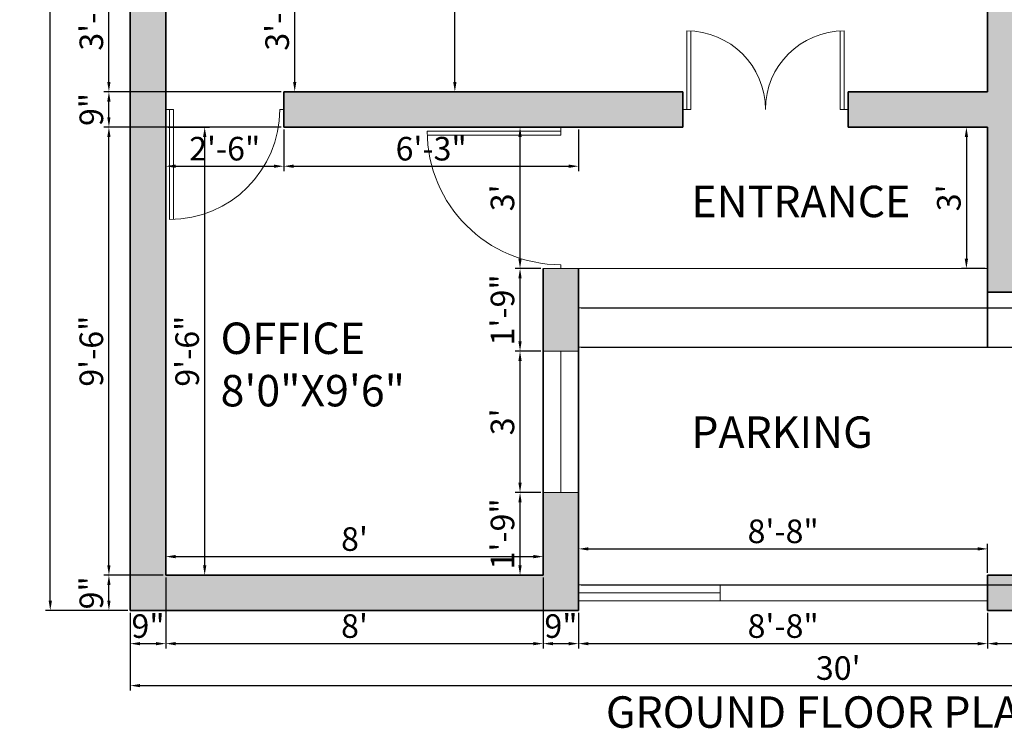
# Model space of a CAD drawing. Units: inches. Extents: x 3592 to 4861, y 1650 to 2243.
# Tile 26 of 30: x 4438 to 4688, y 1655 to 1836. Entities that reach past the tile are written whole.
import ezdxf

# ---------------------------------------------------------------- set-up
doc = ezdxf.new("R2010")
doc.units = ezdxf.units.IN
for name, color, linetype, lineweight in [('A-ANNO-DIMS', 2, 'Continuous', 13), ('A-ANNO-TEXT', 7, 'Continuous', 25), ('A-AREA-IDEN', 7, 'Continuous', 18), ('A-DOOR', 3, 'Continuous', 20), ('A-FLOR-STRS', 7, 'Continuous', 18), ('A-GLAZ', 4, 'Continuous', 18), ('A-WALL', 7, 'Continuous', 35)]:
    doc.layers.add(name, color=color, linetype=linetype, lineweight=lineweight)
doc.layers.add('A-WALL-PATT', color=252, linetype='Continuous', lineweight=13, true_color=0x939598)
doc.styles.get("Standard").update_dxf_attribs({"font": 'arial.ttf'})
doc.dimstyles.new('ISO-25', dxfattribs={"dimtxt": 9, "dimasz": 2.5, "dimexe": 1.25, "dimexo": 0.625, "dimtad": 1, "dimlunit": 3, "dimtxsty": 'Standard', "dimcen": 2.5, "dimadec": 0, "dimazin": 0, "dimtfac": 1, "dimtmove": 0, "dimatfit": 3, "dimfxl": 1, "dimarcsym": 0})

# ---------------------------------------------------------------- blocks, each defined once
blk = doc.blocks.new('2')
for p, q in [((3637.19, 1914.49), (3637.19, 1942.49)), ((3638.19, 1914.49), (3638.19, 1942.49)), ((3636.19, 1914.49), (3638.19, 1914.49)), ((3665.19, 1914.49), (3666.19, 1914.49))]:
    blk.add_line(p, q)
blk.add_arc((3637.19, 1914.49), 28, 0, 90)
blk = doc.blocks.new('1')
for p, q in [((3628.27, 1890.86), (3628.27, 1924.86)), ((3629.27, 1890.86), (3629.27, 1924.86)), ((3627.27, 1890.86), (3629.27, 1890.86)), ((3662.27, 1890.86), (3663.27, 1890.86))]:
    blk.add_line(p, q)
blk.add_arc((3628.27, 1890.86), 34, 0, 90)
blk = doc.blocks.new('MD')
for p, q in [((3665.34, 1831.69), (3665.34, 1851.69)), ((3666.34, 1831.69), (3666.34, 1851.69)), ((3704.34, 1831.69), (3704.34, 1851.69)), ((3705.34, 1831.69), (3705.34, 1851.69)), ((3664.34, 1831.69), (3666.34, 1831.69)), ((3706.34, 1831.69), (3704.34, 1831.69))]:
    blk.add_line(p, q)
for centre, start, end in [((3665.34, 1831.69), 0, 90), ((3705.34, 1831.69), 90, 180)]:
    blk.add_arc(centre, 20, start, end)
blk = doc.blocks.new('*D77')
at = {"layer": 'A-ANNO-DIMS', "color": 0, "lineweight": -2, "transparency": 16777216}
for p, q in [((4475.25, 1694.84), (4475.25, 1700.18)), ((4571.25, 1694.84), (4571.25, 1700.18)), ((4477.75, 1698.93), (4568.75, 1698.93))]:
    blk.add_line(p, q, dxfattribs=at)
at = {"layer": 'A-ANNO-DIMS', "color": 0, "transparency": 16777216}
for points in [[(4477.75, 1699.35), (4477.75, 1698.51), (4475.25, 1698.93)], [(4568.75, 1699.35), (4568.75, 1698.51), (4571.25, 1698.93)]]:
    blk.add_solid(points, dxfattribs=at)
at = {"layer": 'Defpoints', "color": 0, "transparency": 16777216}
for p in [(4571.25, 1698.93), (4475.25, 1694.22), (4571.25, 1694.22)]:
    blk.add_point(p, dxfattribs=at)
at = {"layer": 'A-ANNO-DIMS', "color": 0, "transparency": 16777216, "insert": (4523.25, 1702.62), "char_height": 6, "attachment_point": 5}
blk.add_mtext("8'", dxfattribs=at)
blk = doc.blocks.new('*D78')
at = {"layer": 'A-ANNO-DIMS', "color": 0, "lineweight": -2, "transparency": 16777216}
for p, q in [((4570.62, 1715.22), (4564.1, 1715.22)), ((4565.35, 1696.72), (4565.35, 1712.72)), ((4570.62, 1694.22), (4564.1, 1694.22))]:
    blk.add_line(p, q, dxfattribs=at)
at = {"layer": 'A-ANNO-DIMS', "color": 0, "transparency": 16777216}
for points in [[(4564.93, 1712.72), (4565.76, 1712.72), (4565.35, 1715.22)], [(4564.93, 1696.72), (4565.76, 1696.72), (4565.35, 1694.22)]]:
    blk.add_solid(points, dxfattribs=at)
at = {"layer": 'Defpoints', "color": 0, "transparency": 16777216}
for p in [(4565.35, 1715.22), (4571.25, 1715.22), (4571.25, 1694.22)]:
    blk.add_point(p, dxfattribs=at)
at = {"layer": 'A-ANNO-DIMS', "color": 0, "transparency": 16777216, "insert": (4561.66, 1704.72), "char_height": 6, "attachment_point": 5, "rotation": 90}
blk.add_mtext('1\'-9"', dxfattribs=at)
blk = doc.blocks.new('*D79')
at = {"layer": 'A-ANNO-DIMS', "color": 0, "lineweight": -2, "transparency": 16777216}
for p, q in [((4570.62, 1751.22), (4564.1, 1751.22)), ((4565.35, 1717.72), (4565.35, 1748.72)), ((4570.62, 1715.22), (4564.1, 1715.22))]:
    blk.add_line(p, q, dxfattribs=at)
at = {"layer": 'A-ANNO-DIMS', "color": 0, "transparency": 16777216}
for points in [[(4564.93, 1748.72), (4565.76, 1748.72), (4565.35, 1751.22)], [(4564.93, 1717.72), (4565.76, 1717.72), (4565.35, 1715.22)]]:
    blk.add_solid(points, dxfattribs=at)
at = {"layer": 'Defpoints', "color": 0, "transparency": 16777216}
for p in [(4565.35, 1751.22), (4571.25, 1751.22), (4571.25, 1715.22)]:
    blk.add_point(p, dxfattribs=at)
at = {"layer": 'A-ANNO-DIMS', "color": 0, "transparency": 16777216, "insert": (4561.66, 1733.22), "char_height": 6, "attachment_point": 5, "rotation": 90}
blk.add_mtext("3'", dxfattribs=at)
blk = doc.blocks.new('*D80')
at = {"layer": 'A-ANNO-DIMS', "color": 0, "lineweight": -2, "transparency": 16777216}
for p, q in [((4570.62, 1772.22), (4564.1, 1772.22)), ((4565.35, 1753.72), (4565.35, 1769.72)), ((4570.62, 1751.22), (4564.1, 1751.22))]:
    blk.add_line(p, q, dxfattribs=at)
at = {"layer": 'A-ANNO-DIMS', "color": 0, "transparency": 16777216}
for points in [[(4564.93, 1769.72), (4565.76, 1769.72), (4565.35, 1772.22)], [(4564.93, 1753.72), (4565.76, 1753.72), (4565.35, 1751.22)]]:
    blk.add_solid(points, dxfattribs=at)
at = {"layer": 'Defpoints', "color": 0, "transparency": 16777216}
for p in [(4565.35, 1772.22), (4571.25, 1772.22), (4571.25, 1751.22)]:
    blk.add_point(p, dxfattribs=at)
at = {"layer": 'A-ANNO-DIMS', "color": 0, "transparency": 16777216, "insert": (4561.66, 1761.72), "char_height": 6, "attachment_point": 5, "rotation": 90}
blk.add_mtext('1\'-9"', dxfattribs=at)
blk = doc.blocks.new('*D81')
at = {"layer": 'A-ANNO-DIMS', "color": 0, "lineweight": -2, "transparency": 16777216}
for p, q in [((4565.97, 1808.22), (4566.6, 1808.22)), ((4565.35, 1774.72), (4565.35, 1805.72)), ((4570.62, 1772.22), (4564.1, 1772.22))]:
    blk.add_line(p, q, dxfattribs=at)
at = {"layer": 'A-ANNO-DIMS', "color": 0, "transparency": 16777216}
for points in [[(4564.93, 1805.72), (4565.76, 1805.72), (4565.35, 1808.22)], [(4564.93, 1774.72), (4565.76, 1774.72), (4565.35, 1772.22)]]:
    blk.add_solid(points, dxfattribs=at)
at = {"layer": 'Defpoints', "color": 0, "transparency": 16777216}
for p in [(4565.35, 1808.22), (4565.35, 1808.22), (4571.25, 1772.22)]:
    blk.add_point(p, dxfattribs=at)
at = {"layer": 'A-ANNO-DIMS', "color": 0, "transparency": 16777216, "insert": (4561.66, 1790.22), "char_height": 6, "attachment_point": 5, "rotation": 90}
blk.add_mtext("3'", dxfattribs=at)
blk = doc.blocks.new('*D82')
at = {"layer": 'A-ANNO-DIMS', "color": 0, "lineweight": -2, "transparency": 16777216}
for p, q in [((4475.25, 1807.59), (4475.25, 1797.02)), ((4505.25, 1807.59), (4505.25, 1797.02)), ((4477.75, 1798.27), (4502.75, 1798.27))]:
    blk.add_line(p, q, dxfattribs=at)
at = {"layer": 'A-ANNO-DIMS', "color": 0, "transparency": 16777216}
for points in [[(4477.75, 1798.69), (4477.75, 1797.86), (4475.25, 1798.27)], [(4502.75, 1798.69), (4502.75, 1797.86), (4505.25, 1798.27)]]:
    blk.add_solid(points, dxfattribs=at)
at = {"layer": 'Defpoints', "color": 0, "transparency": 16777216}
for p in [(4475.25, 1808.22), (4505.25, 1808.22), (4505.25, 1798.27)]:
    blk.add_point(p, dxfattribs=at)
at = {"layer": 'A-ANNO-DIMS', "color": 0, "transparency": 16777216, "insert": (4490.25, 1801.96), "char_height": 6, "attachment_point": 5}
blk.add_mtext('2\'-6"', dxfattribs=at)
blk = doc.blocks.new('*D83')
at = {"layer": 'A-ANNO-DIMS', "color": 0, "lineweight": -2, "transparency": 16777216}
for p, q in [((4505.25, 1807.59), (4505.25, 1797.02)), ((4580.25, 1807.59), (4580.25, 1797.02)), ((4507.75, 1798.27), (4577.75, 1798.27))]:
    blk.add_line(p, q, dxfattribs=at)
at = {"layer": 'A-ANNO-DIMS', "color": 0, "transparency": 16777216}
for points in [[(4507.75, 1798.69), (4507.75, 1797.86), (4505.25, 1798.27)], [(4577.75, 1798.69), (4577.75, 1797.86), (4580.25, 1798.27)]]:
    blk.add_solid(points, dxfattribs=at)
at = {"layer": 'Defpoints', "color": 0, "transparency": 16777216}
for p in [(4505.25, 1808.22), (4580.25, 1808.22), (4580.25, 1798.27)]:
    blk.add_point(p, dxfattribs=at)
at = {"layer": 'A-ANNO-DIMS', "color": 0, "transparency": 16777216, "insert": (4542.75, 1801.96), "char_height": 6, "attachment_point": 5}
blk.add_mtext('6\'-3"', dxfattribs=at)
blk = doc.blocks.new('*D84')
at = {"layer": 'A-ANNO-DIMS', "color": 0, "lineweight": -2, "transparency": 16777216}
for p, q in [((4475.87, 1808.22), (4486.42, 1808.22)), ((4485.17, 1696.72), (4485.17, 1805.72)), ((4475.87, 1694.22), (4486.42, 1694.22))]:
    blk.add_line(p, q, dxfattribs=at)
at = {"layer": 'A-ANNO-DIMS', "color": 0, "transparency": 16777216}
for points in [[(4484.75, 1805.72), (4485.59, 1805.72), (4485.17, 1808.22)], [(4484.75, 1696.72), (4485.59, 1696.72), (4485.17, 1694.22)]]:
    blk.add_solid(points, dxfattribs=at)
at = {"layer": 'Defpoints', "color": 0, "transparency": 16777216}
for p in [(4475.25, 1808.22), (4485.17, 1808.22), (4475.25, 1694.22)]:
    blk.add_point(p, dxfattribs=at)
at = {"layer": 'A-ANNO-DIMS', "color": 0, "transparency": 16777216, "insert": (4481.48, 1751.22), "char_height": 6, "attachment_point": 5, "rotation": 90}
blk.add_mtext('9\'-6"', dxfattribs=at)
blk = doc.blocks.new('*D85')
at = {"layer": 'A-ANNO-DIMS', "color": 0, "lineweight": -2, "transparency": 16777216}
for p, q in [((4505.87, 1856.22), (4509.31, 1856.22)), ((4508.06, 1819.72), (4508.06, 1853.72)), ((4505.87, 1817.22), (4509.31, 1817.22))]:
    blk.add_line(p, q, dxfattribs=at)
at = {"layer": 'A-ANNO-DIMS', "color": 0, "transparency": 16777216}
for points in [[(4507.64, 1853.72), (4508.47, 1853.72), (4508.06, 1856.22)], [(4507.64, 1819.72), (4508.47, 1819.72), (4508.06, 1817.22)]]:
    blk.add_solid(points, dxfattribs=at)
at = {"layer": 'Defpoints', "color": 0, "transparency": 16777216}
for p in [(4505.25, 1856.22), (4508.06, 1856.22), (4505.25, 1817.22)]:
    blk.add_point(p, dxfattribs=at)
at = {"layer": 'A-ANNO-DIMS', "color": 0, "transparency": 16777216, "insert": (4504.37, 1836.72), "char_height": 6, "attachment_point": 5, "rotation": 90}
blk.add_mtext('3\'-3"', dxfattribs=at)
blk = doc.blocks.new('*D92')
at = {"layer": 'A-ANNO-DIMS', "color": 0, "lineweight": -2, "transparency": 16777216}
for p, q in [((4546.11, 2020.22), (4550.03, 2020.22)), ((4548.78, 1819.72), (4548.78, 2017.72)), ((4546.11, 1817.22), (4550.03, 1817.22))]:
    blk.add_line(p, q, dxfattribs=at)
at = {"layer": 'A-ANNO-DIMS', "color": 0, "transparency": 16777216}
for points in [[(4548.36, 2017.72), (4549.19, 2017.72), (4548.78, 2020.22)], [(4548.36, 1819.72), (4549.19, 1819.72), (4548.78, 1817.22)]]:
    blk.add_solid(points, dxfattribs=at)
at = {"layer": 'Defpoints', "color": 0, "transparency": 16777216}
for p in [(4545.48, 2020.22), (4548.78, 2020.22), (4545.48, 1817.22)]:
    blk.add_point(p, dxfattribs=at)
at = {"layer": 'A-ANNO-DIMS', "color": 0, "transparency": 16777216, "insert": (4545.09, 1918.72), "char_height": 6, "attachment_point": 5, "rotation": 90}
blk.add_mtext('16\'-11"', dxfattribs=at)
blk = doc.blocks.new('*D94')
at = {"layer": 'A-ANNO-DIMS', "color": 0, "lineweight": -2, "transparency": 16777216}
for p, q in [((4475.25, 1693.59), (4475.25, 1675.54)), ((4466.25, 1684.59), (4466.25, 1675.54)), ((4468.75, 1676.79), (4472.75, 1676.79))]:
    blk.add_line(p, q, dxfattribs=at)
at = {"layer": 'A-ANNO-DIMS', "color": 0, "transparency": 16777216}
for points in [[(4468.75, 1677.2), (4468.75, 1676.37), (4466.25, 1676.79)], [(4472.75, 1677.2), (4472.75, 1676.37), (4475.25, 1676.79)]]:
    blk.add_solid(points, dxfattribs=at)
at = {"layer": 'Defpoints', "color": 0, "transparency": 16777216}
for p in [(4475.25, 1694.22), (4466.25, 1685.22), (4475.25, 1676.79)]:
    blk.add_point(p, dxfattribs=at)
at = {"layer": 'A-ANNO-DIMS', "color": 0, "transparency": 16777216, "insert": (4470.75, 1680.48), "char_height": 6, "attachment_point": 5}
blk.add_mtext('9"', dxfattribs=at)
blk = doc.blocks.new('*D95')
at = {"layer": 'A-ANNO-DIMS', "color": 0, "lineweight": -2, "transparency": 16777216}
for p, q in [((4475.25, 1693.59), (4475.25, 1675.54)), ((4571.25, 1693.59), (4571.25, 1675.54)), ((4477.75, 1676.79), (4568.75, 1676.79))]:
    blk.add_line(p, q, dxfattribs=at)
at = {"layer": 'A-ANNO-DIMS', "color": 0, "transparency": 16777216}
for points in [[(4477.75, 1677.2), (4477.75, 1676.37), (4475.25, 1676.79)], [(4568.75, 1677.2), (4568.75, 1676.37), (4571.25, 1676.79)]]:
    blk.add_solid(points, dxfattribs=at)
at = {"layer": 'Defpoints', "color": 0, "transparency": 16777216}
for p in [(4475.25, 1694.22), (4571.25, 1694.22), (4571.25, 1676.79)]:
    blk.add_point(p, dxfattribs=at)
at = {"layer": 'A-ANNO-DIMS', "color": 0, "transparency": 16777216, "insert": (4523.25, 1680.48), "char_height": 6, "attachment_point": 5}
blk.add_mtext("8'", dxfattribs=at)
blk = doc.blocks.new('*D96')
at = {"layer": 'A-ANNO-DIMS', "color": 0, "lineweight": -2, "transparency": 16777216}
for p, q in [((4571.25, 1693.59), (4571.25, 1675.54)), ((4580.25, 1684.59), (4580.25, 1675.54)), ((4573.75, 1676.79), (4577.75, 1676.79))]:
    blk.add_line(p, q, dxfattribs=at)
at = {"layer": 'A-ANNO-DIMS', "color": 0, "transparency": 16777216}
for points in [[(4573.75, 1677.2), (4573.75, 1676.37), (4571.25, 1676.79)], [(4577.75, 1677.2), (4577.75, 1676.37), (4580.25, 1676.79)]]:
    blk.add_solid(points, dxfattribs=at)
at = {"layer": 'Defpoints', "color": 0, "transparency": 16777216}
for p in [(4571.25, 1694.22), (4580.25, 1685.22), (4580.25, 1676.79)]:
    blk.add_point(p, dxfattribs=at)
at = {"layer": 'A-ANNO-DIMS', "color": 0, "transparency": 16777216, "insert": (4575.75, 1680.48), "char_height": 6, "attachment_point": 5}
blk.add_mtext('9"', dxfattribs=at)
blk = doc.blocks.new('*D97')
at = {"layer": 'A-ANNO-DIMS', "color": 0, "lineweight": -2, "transparency": 16777216}
for p, q in [((4580.25, 1684.59), (4580.25, 1675.54)), ((4684.25, 1684.59), (4684.25, 1675.54)), ((4582.75, 1676.79), (4681.75, 1676.79))]:
    blk.add_line(p, q, dxfattribs=at)
at = {"layer": 'A-ANNO-DIMS', "color": 0, "transparency": 16777216}
for points in [[(4582.75, 1677.2), (4582.75, 1676.37), (4580.25, 1676.79)], [(4681.75, 1677.2), (4681.75, 1676.37), (4684.25, 1676.79)]]:
    blk.add_solid(points, dxfattribs=at)
at = {"layer": 'Defpoints', "color": 0, "transparency": 16777216}
for p in [(4580.25, 1685.22), (4684.25, 1685.22), (4684.25, 1676.79)]:
    blk.add_point(p, dxfattribs=at)
at = {"layer": 'A-ANNO-DIMS', "color": 0, "transparency": 16777216, "insert": (4632.25, 1680.48), "char_height": 6, "attachment_point": 5}
blk.add_mtext('8\'-8"', dxfattribs=at)
blk = doc.blocks.new('*D98')
at = {"layer": 'A-ANNO-DIMS', "color": 0, "lineweight": -2, "transparency": 16777216}
for p, q in [((4817.25, 1693.59), (4817.25, 1675.54)), ((4684.25, 1684.59), (4684.25, 1675.54)), ((4686.75, 1676.79), (4814.75, 1676.79))]:
    blk.add_line(p, q, dxfattribs=at)
at = {"layer": 'A-ANNO-DIMS', "color": 0, "transparency": 16777216}
for points in [[(4686.75, 1677.2), (4686.75, 1676.37), (4684.25, 1676.79)], [(4814.75, 1677.2), (4814.75, 1676.37), (4817.25, 1676.79)]]:
    blk.add_solid(points, dxfattribs=at)
at = {"layer": 'Defpoints', "color": 0, "transparency": 16777216}
for p in [(4817.25, 1694.22), (4684.25, 1685.22), (4817.25, 1676.79)]:
    blk.add_point(p, dxfattribs=at)
at = {"layer": 'A-ANNO-DIMS', "color": 0, "transparency": 16777216, "insert": (4750.75, 1680.42), "char_height": 6, "attachment_point": 5}
blk.add_mtext('11\'-1"', dxfattribs=at)
blk = doc.blocks.new('*D100')
at = {"layer": 'A-ANNO-DIMS', "color": 0, "lineweight": -2, "transparency": 16777216}
for p, q in [((4474.62, 1694.22), (4459.56, 1694.22)), ((4460.81, 1687.72), (4460.81, 1691.72)), ((4465.62, 1685.22), (4459.56, 1685.22))]:
    blk.add_line(p, q, dxfattribs=at)
at = {"layer": 'A-ANNO-DIMS', "color": 0, "transparency": 16777216}
for points in [[(4460.39, 1691.72), (4461.22, 1691.72), (4460.81, 1694.22)], [(4460.39, 1687.72), (4461.22, 1687.72), (4460.81, 1685.22)]]:
    blk.add_solid(points, dxfattribs=at)
at = {"layer": 'Defpoints', "color": 0, "transparency": 16777216}
for p in [(4460.81, 1694.22), (4475.25, 1694.22), (4466.25, 1685.22)]:
    blk.add_point(p, dxfattribs=at)
at = {"layer": 'A-ANNO-DIMS', "color": 0, "transparency": 16777216, "insert": (4457.12, 1689.72), "char_height": 6, "attachment_point": 5, "rotation": 90}
blk.add_mtext('9"', dxfattribs=at)
blk = doc.blocks.new('*D101')
at = {"layer": 'A-ANNO-DIMS', "color": 0, "lineweight": -2, "transparency": 16777216}
for p, q in [((4504.62, 1808.22), (4459.56, 1808.22)), ((4460.81, 1696.72), (4460.81, 1805.72)), ((4474.62, 1694.22), (4459.56, 1694.22))]:
    blk.add_line(p, q, dxfattribs=at)
at = {"layer": 'A-ANNO-DIMS', "color": 0, "transparency": 16777216}
for points in [[(4460.39, 1805.72), (4461.22, 1805.72), (4460.81, 1808.22)], [(4460.39, 1696.72), (4461.22, 1696.72), (4460.81, 1694.22)]]:
    blk.add_solid(points, dxfattribs=at)
at = {"layer": 'Defpoints', "color": 0, "transparency": 16777216}
for p in [(4460.81, 1808.22), (4505.25, 1808.22), (4475.25, 1694.22)]:
    blk.add_point(p, dxfattribs=at)
at = {"layer": 'A-ANNO-DIMS', "color": 0, "transparency": 16777216, "insert": (4457.12, 1751.22), "char_height": 6, "attachment_point": 5, "rotation": 90}
blk.add_mtext('9\'-6"', dxfattribs=at)
blk = doc.blocks.new('*D102')
at = {"layer": 'A-ANNO-DIMS', "color": 0, "lineweight": -2, "transparency": 16777216}
for p, q in [((4504.62, 1817.22), (4459.56, 1817.22)), ((4460.81, 1810.72), (4460.81, 1814.72)), ((4504.62, 1808.22), (4459.56, 1808.22))]:
    blk.add_line(p, q, dxfattribs=at)
at = {"layer": 'A-ANNO-DIMS', "color": 0, "transparency": 16777216}
for points in [[(4460.39, 1814.72), (4461.22, 1814.72), (4460.81, 1817.22)], [(4460.39, 1810.72), (4461.22, 1810.72), (4460.81, 1808.22)]]:
    blk.add_solid(points, dxfattribs=at)
at = {"layer": 'Defpoints', "color": 0, "transparency": 16777216}
for p in [(4460.81, 1817.22), (4505.25, 1817.22), (4505.25, 1808.22)]:
    blk.add_point(p, dxfattribs=at)
at = {"layer": 'A-ANNO-DIMS', "color": 0, "transparency": 16777216, "insert": (4457.12, 1812.72), "char_height": 6, "attachment_point": 5, "rotation": 90}
blk.add_mtext('9"', dxfattribs=at)
blk = doc.blocks.new('*D103')
at = {"layer": 'A-ANNO-DIMS', "color": 0, "lineweight": -2, "transparency": 16777216}
for p, q in [((4504.62, 1856.22), (4459.56, 1856.22)), ((4460.81, 1819.72), (4460.81, 1853.72)), ((4504.62, 1817.22), (4459.56, 1817.22))]:
    blk.add_line(p, q, dxfattribs=at)
at = {"layer": 'A-ANNO-DIMS', "color": 0, "transparency": 16777216}
for points in [[(4460.39, 1853.72), (4461.22, 1853.72), (4460.81, 1856.22)], [(4460.39, 1819.72), (4461.22, 1819.72), (4460.81, 1817.22)]]:
    blk.add_solid(points, dxfattribs=at)
at = {"layer": 'Defpoints', "color": 0, "transparency": 16777216}
for p in [(4460.81, 1856.22), (4505.25, 1856.22), (4505.25, 1817.22)]:
    blk.add_point(p, dxfattribs=at)
at = {"layer": 'A-ANNO-DIMS', "color": 0, "transparency": 16777216, "insert": (4457.12, 1836.72), "char_height": 6, "attachment_point": 5, "rotation": 90}
blk.add_mtext('3\'-3"', dxfattribs=at)
blk = doc.blocks.new('*D127')
at = {"layer": 'A-ANNO-DIMS', "color": 0, "lineweight": -2, "transparency": 16777216}
for p, q in [((4466.25, 1684.59), (4466.25, 1664.86)), ((4826.25, 1684.59), (4826.25, 1664.86)), ((4468.75, 1666.11), (4823.75, 1666.11))]:
    blk.add_line(p, q, dxfattribs=at)
at = {"layer": 'A-ANNO-DIMS', "color": 0, "transparency": 16777216}
for points in [[(4468.75, 1666.53), (4468.75, 1665.69), (4466.25, 1666.11)], [(4823.75, 1666.53), (4823.75, 1665.69), (4826.25, 1666.11)]]:
    blk.add_solid(points, dxfattribs=at)
at = {"layer": 'Defpoints', "color": 0, "transparency": 16777216}
for p in [(4466.25, 1685.22), (4826.25, 1685.22), (4826.25, 1666.11)]:
    blk.add_point(p, dxfattribs=at)
at = {"layer": 'A-ANNO-DIMS', "color": 0, "transparency": 16777216, "insert": (4646.25, 1669.8), "char_height": 6, "attachment_point": 5}
blk.add_mtext("30'", dxfattribs=at)
blk = doc.blocks.new('*D128')
at = {"layer": 'A-ANNO-DIMS', "color": 0, "lineweight": -2, "transparency": 16777216}
for p, q in [((4580.25, 1698.04), (4580.25, 1702.15)), ((4582.75, 1700.9), (4681.75, 1700.9)), ((4684.25, 1694.84), (4684.25, 1702.15))]:
    blk.add_line(p, q, dxfattribs=at)
at = {"layer": 'A-ANNO-DIMS', "color": 0, "transparency": 16777216}
for points in [[(4582.75, 1701.32), (4582.75, 1700.49), (4580.25, 1700.9)], [(4681.75, 1701.32), (4681.75, 1700.49), (4684.25, 1700.9)]]:
    blk.add_solid(points, dxfattribs=at)
at = {"layer": 'Defpoints', "color": 0, "transparency": 16777216}
for p in [(4684.25, 1700.9), (4580.25, 1697.41), (4684.25, 1694.22)]:
    blk.add_point(p, dxfattribs=at)
at = {"layer": 'A-ANNO-DIMS', "color": 0, "transparency": 16777216, "insert": (4632.25, 1704.59), "char_height": 6, "attachment_point": 5}
blk.add_mtext('8\'-8"', dxfattribs=at)
blk = doc.blocks.new('*D130')
at = {"layer": 'A-ANNO-DIMS', "color": 0, "lineweight": -2, "transparency": 16777216}
for p, q in [((4683.62, 1808.22), (4677.6, 1808.22)), ((4678.85, 1805.72), (4678.85, 1774.72)), ((4683.62, 1772.22), (4677.6, 1772.22))]:
    blk.add_line(p, q, dxfattribs=at)
at = {"layer": 'A-ANNO-DIMS', "color": 0, "transparency": 16777216}
for points in [[(4678.43, 1805.72), (4679.27, 1805.72), (4678.85, 1808.22)], [(4678.43, 1774.72), (4679.27, 1774.72), (4678.85, 1772.22)]]:
    blk.add_solid(points, dxfattribs=at)
at = {"layer": 'Defpoints', "color": 0, "transparency": 16777216}
for p in [(4684.25, 1808.22), (4678.85, 1772.22), (4684.25, 1772.22)]:
    blk.add_point(p, dxfattribs=at)
at = {"layer": 'A-ANNO-DIMS', "color": 0, "transparency": 16777216, "insert": (4675.16, 1790.22), "char_height": 6, "attachment_point": 5, "rotation": 90}
blk.add_mtext("3'", dxfattribs=at)
blk = doc.blocks.new('*D131')
at = {"layer": 'A-ANNO-DIMS', "color": 0, "lineweight": -2, "transparency": 16777216}
for p, q in [((4465.62, 2165.22), (4444.65, 2165.22)), ((4445.9, 1687.72), (4445.9, 2162.72)), ((4465.62, 1685.22), (4444.65, 1685.22))]:
    blk.add_line(p, q, dxfattribs=at)
at = {"layer": 'A-ANNO-DIMS', "color": 0, "transparency": 16777216}
for points in [[(4445.49, 2162.72), (4446.32, 2162.72), (4445.9, 2165.22)], [(4445.49, 1687.72), (4446.32, 1687.72), (4445.9, 1685.22)]]:
    blk.add_solid(points, dxfattribs=at)
at = {"layer": 'Defpoints', "color": 0, "transparency": 16777216}
for p in [(4445.9, 2165.22), (4466.25, 2165.22), (4466.25, 1685.22)]:
    blk.add_point(p, dxfattribs=at)
at = {"layer": 'A-ANNO-DIMS', "color": 0, "transparency": 16777216, "insert": (4442.21, 1925.22), "char_height": 6, "attachment_point": 5, "rotation": 90}
blk.add_mtext("40'", dxfattribs=at)
blk = doc.blocks.new('GATE-PARKING-104')
for p, q in [((104, 4), (0, 4)), ((36, 0), (36, 4)), ((36, 2), (0, 2)), ((104, 0), (0, 0))]:
    blk.add_line(p, q)
blk = doc.blocks.new('*D183')
at = {"layer": 'A-ANNO-DIMS', "color": 0, "lineweight": -2, "transparency": 16777216}
for p, q in [((4853.35, 1762.22), (4853.35, 1796.89)), ((4580.87, 1762.22), (4854.6, 1762.22)), ((4853.35, 1754.72), (4853.35, 1759.72)), ((4580.87, 1752.22), (4854.6, 1752.22))]:
    blk.add_line(p, q, dxfattribs=at)
at = {"layer": 'A-ANNO-DIMS', "color": 0, "transparency": 16777216}
for points in [[(4852.93, 1759.72), (4853.77, 1759.72), (4853.35, 1762.22)], [(4852.93, 1754.72), (4853.77, 1754.72), (4853.35, 1752.22)]]:
    blk.add_solid(points, dxfattribs=at)
at = {"layer": 'Defpoints', "color": 0, "transparency": 16777216}
for p in [(4580.25, 1762.22), (4853.35, 1762.22), (4580.25, 1752.22)]:
    blk.add_point(p, dxfattribs=at)
at = {"layer": 'A-ANNO-DIMS', "color": 0, "transparency": 16777216, "insert": (4848.13, 1780.8), "char_height": 9, "attachment_point": 5, "rotation": 90}
blk.add_mtext('0\'-10"', dxfattribs=at)
blk = doc.blocks.new('*D184')
at = {"layer": 'A-ANNO-DIMS', "color": 0, "lineweight": -2, "transparency": 16777216}
for p, q in [((4580.87, 1752.22), (4854.6, 1752.22)), ((4853.35, 1694.22), (4853.35, 1749.72)), ((4580.87, 1691.72), (4854.6, 1691.72))]:
    blk.add_line(p, q, dxfattribs=at)
at = {"layer": 'A-ANNO-DIMS', "color": 0, "transparency": 16777216}
for points in [[(4852.93, 1749.72), (4853.77, 1749.72), (4853.35, 1752.22)], [(4852.93, 1694.22), (4853.77, 1694.22), (4853.35, 1691.72)]]:
    blk.add_solid(points, dxfattribs=at)
at = {"layer": 'Defpoints', "color": 0, "transparency": 16777216}
for p in [(4580.25, 1752.22), (4853.35, 1752.22), (4580.25, 1691.72)]:
    blk.add_point(p, dxfattribs=at)
at = {"layer": 'A-ANNO-DIMS', "color": 0, "transparency": 16777216, "insert": (4848.07, 1721.97), "char_height": 9, "attachment_point": 5, "rotation": 90}
blk.add_mtext('5\'-0 1/2"', dxfattribs=at)

msp = doc.modelspace()

# ---------------------------------------------------------------- hatches: boundary and pattern name
at = {"layer": 'A-WALL-PATT'}
h = msp.add_hatch(color=256, dxfattribs=at)
h.dxf.hatch_style = 1
h.paths.add_polyline_path([(4466.25, 2165.219), (4466.25, 1993.219), (4475.25, 1993.219), (4475.25, 2156.219), (4619.25, 2156.219), (4619.25, 2150.219), (4623.25, 2150.219), (4623.25, 2156.219), (4684.25, 2156.219), (4684.25, 2150.219), (4693.25, 2150.219), (4693.25, 2156.219), (4817.25, 2156.219), (4817.25, 2114.219), (4826.25, 2114.219), (4826.25, 2165.219)])
h.paths.add_polyline_path([(4623.25, 2096.219), (4623.25, 2102.219), (4619.25, 2102.219), (4619.25, 2020.219), (4623.25, 2020.219), (4623.25, 2087.219), (4684.25, 2087.219), (4684.25, 2020.219), (4734.25, 2020.219), (4734.25, 2024.219), (4693.25, 2024.219), (4693.25, 2102.219), (4684.25, 2102.219), (4684.25, 2096.219)], flags=17)
h.paths.add_polyline_path([(4817.25, 2024.219), (4776.25, 2024.219), (4776.25, 2020.219), (4817.25, 2020.219), (4817.25, 1989.719), (4826.25, 1989.719), (4826.25, 2066.219), (4817.25, 2066.219)])
h.paths.add_polyline_path([(4817.25, 1865.219), (4826.25, 1865.219), (4826.25, 1941.719), (4817.25, 1941.719), (4817.25, 1911.219), (4729.25, 1911.219), (4729.25, 1907.219), (4817.25, 1907.219)])
h.paths.add_polyline_path([(4826.25, 1817.219), (4817.25, 1817.219), (4817.25, 1775.219), (4693.25, 1775.219), (4693.25, 1911.219), (4684.25, 1911.219), (4684.25, 1817.219), (4648.75, 1817.219), (4648.75, 1808.219), (4684.25, 1808.219), (4684.25, 1766.219), (4817.25, 1766.219), (4817.25, 1694.219), (4684.25, 1694.219), (4684.25, 1685.219), (4826.25, 1685.219)])
h.paths.add_polyline_path([(4505.25, 1817.219), (4505.25, 1808.219), (4606.75, 1808.219), (4606.75, 1817.219)])
h.paths.add_polyline_path([(4539.25, 1856.219), (4539.25, 2020.219), (4583.25, 2020.219), (4583.25, 2024.219), (4505.25, 2024.219), (4505.25, 2020.219), (4535.25, 2020.219), (4535.25, 1942.219), (4475.25, 1942.219), (4475.25, 1969.219), (4466.25, 1969.219), (4466.25, 1911.219), (4475.25, 1911.219), (4475.25, 1938.219), (4535.25, 1938.219), (4535.25, 1860.219), (4505.25, 1860.219), (4505.25, 1856.219)])
h.paths.add_polyline_path([(4475.25, 1887.219), (4466.25, 1887.219), (4466.25, 1685.219), (4580.25, 1685.219), (4580.25, 1715.219), (4571.25, 1715.219), (4571.25, 1694.219), (4475.25, 1694.219)])
h.paths.add_polyline_path([(4571.25, 1751.219), (4580.25, 1751.219), (4580.25, 1772.219), (4571.25, 1772.219)], flags=17)

# ---------------------------------------------------------------- linework, layer by layer
at = {"layer": 'A-FLOR-STRS'}
for p, q in [((4684.25, 1772.219), (4571.25, 1772.219)), ((4684.25, 1762.219), (4580.25, 1762.219)), ((4684.25, 1752.219), (4580.25, 1752.219))]:
    msp.add_line(p, q, dxfattribs=at)
at = {"layer": 'A-GLAZ'}
for p, q in [((4571.25, 1751.219), (4580.25, 1751.219)), ((4575.75, 1751.219), (4575.75, 1715.219)), ((4571.25, 1715.219), (4580.25, 1715.219))]:
    msp.add_line(p, q, dxfattribs=at)
at = {"layer": 'A-WALL'}
for p, q in [((4466.25, 1685.219), (4466.25, 2165.219)), ((4475.25, 1694.219), (4475.25, 1938.219)), ((4684.25, 1911.219), (4684.25, 1817.219)), ((4606.75, 1817.219), (4505.25, 1817.219)), ((4505.25, 1808.219), (4505.25, 1817.219)), ((4606.75, 1808.219), (4606.75, 1817.219)), ((4684.25, 1817.219), (4648.75, 1817.219)), ((4648.75, 1808.219), (4648.75, 1817.219)), ((4606.75, 1808.219), (4505.25, 1808.219)), ((4684.25, 1808.219), (4648.75, 1808.219)), ((4684.25, 1808.219), (4684.25, 1752.219)), ((4571.25, 1694.219), (4571.25, 1772.219)), ((4580.25, 1685.219), (4580.25, 1772.219)), ((4817.25, 1766.219), (4684.25, 1766.219)), ((4571.25, 1694.219), (4475.25, 1694.219)), ((4684.25, 1694.219), (4684.25, 1685.219)), ((4817.25, 1694.219), (4684.25, 1694.219)), ((4580.25, 1685.219), (4466.25, 1685.219)), ((4826.25, 1685.219), (4684.25, 1685.219))]:
    msp.add_line(p, q, dxfattribs=at)

# ---------------------------------------------------------------- block references
at = {"layer": 'A-DOOR'}
for name, p in [('MD', (942.414, -18.97)), ('GATE-PARKING-104', (4580.249, 1687.719))]:
    msp.add_blockref(name, p, dxfattribs=at)
at = {"layer": 'A-DOOR', "xscale": -1}
for name, p, rotation in [('2', (839.061, 3727.211), 180), ('1', (6466.614, 5435.486), 90)]:
    msp.add_blockref(name, p, dxfattribs=dict(at, rotation=rotation))

# ---------------------------------------------------------------- texts
at = {"layer": 'A-ANNO-TEXT', "insert": (4587.182, 1663.381), "char_height": 8, "attachment_point": 1}
msp.add_mtext_dynamic_manual_height_columns('GROUND FLOOR PLAN', width=131.60551, gutter_width=12.5, heights=[0], dxfattribs=at)
at = {"layer": 'A-AREA-IDEN', "char_height": 8, "attachment_point": 1}
for s, insert in [('ENTRANCE', (4608.895, 1793.311)), ('OFFICE\\P8\'0"X9\'6"', (4489.201, 1758.494)), ('PARKING', (4608.895, 1734.612))]:
    msp.add_mtext_dynamic_manual_height_columns(s, width=121.44943, gutter_width=12.5, heights=[0], dxfattribs=dict(at, insert=insert))

# ---------------------------------------------------------------- dimensions: what is measured, and where the dimension line sits
at = {"layer": 'A-ANNO-DIMS'}
for base, p1, p2, override, picture, middle in [((4445.902, 2165.219), (4466.25, 1685.219), (4466.25, 2165.219), {"dimtxt": 6, "dimclrd": 0, "dimclre": 0, "dimclrt": 0}, '*D131', (4442.214, 1925.219)), ((4548.776, 2020.219), (4545.484, 1817.219), (4545.484, 2020.219), {"dimtxt": 6, "dimclrd": 0, "dimclre": 0, "dimclrt": 0}, '*D92', (4545.088, 1918.719)), ((4460.807, 1856.219), (4505.25, 1817.219), (4505.25, 1856.219), {"dimtxt": 6, "dimclrd": 0, "dimclre": 0, "dimclrt": 0, "dimtmove": 1}, '*D103', (4457.116, 1836.719)), ((4508.058, 1856.219), (4505.25, 1817.219), (4505.25, 1856.219), {"dimtxt": 6, "dimclrd": 0, "dimclre": 0, "dimclrt": 0}, '*D85', (4504.368, 1836.719)), ((4460.807, 1817.219), (4505.25, 1808.219), (4505.25, 1817.219), {"dimtxt": 6, "dimclrd": 0, "dimclre": 0, "dimclrt": 0, "dimtmove": 1}, '*D102', (4457.118, 1812.719)), ((4460.807, 1808.219), (4475.25, 1694.219), (4505.25, 1808.219), {"dimtxt": 6, "dimclrd": 0, "dimclre": 0, "dimclrt": 0, "dimtmove": 1}, '*D101', (4457.118, 1751.219)), ((4485.17, 1808.219), (4475.25, 1694.219), (4475.25, 1808.219), {"dimtxt": 6, "dimclrd": 0, "dimclre": 0, "dimclrt": 0}, '*D84', (4481.481, 1751.219)), ((4565.348, 1808.219), (4571.25, 1772.219), (4565.348, 1808.219), {"dimtxt": 6, "dimclrd": 0, "dimclre": 0, "dimclrt": 0, "dimtmove": 1}, '*D81', (4561.657, 1790.219)), ((4678.851, 1772.219), (4684.25, 1808.219), (4684.25, 1772.219), {"dimtxt": 6, "dimclrd": 0, "dimclre": 0, "dimclrt": 0}, '*D130', (4675.161, 1790.219)), ((4853.35, 1762.219), (4580.25, 1752.219), (4580.25, 1762.219), {"dimdec": 1, "dimlfac": 1, "dimrnd": 0, "dimzin": 1, "dimdsep": 46, "dimlunit": 4, "dimfrac": 2}, '*D183', (4848.13, 1780.802)), ((4565.348, 1772.219), (4571.25, 1751.219), (4571.25, 1772.219), {"dimtxt": 6, "dimclrd": 0, "dimclre": 0, "dimclrt": 0, "dimtmove": 1}, '*D80', (4561.659, 1761.719)), ((4565.348, 1751.219), (4571.25, 1715.219), (4571.25, 1751.219), {"dimtxt": 6, "dimclrd": 0, "dimclre": 0, "dimclrt": 0, "dimtmove": 1}, '*D79', (4561.657, 1733.219)), ((4853.35, 1752.219), (4580.25, 1691.719), (4580.25, 1752.219), {"dimdec": 1, "dimlfac": 1, "dimrnd": 0, "dimzin": 1, "dimdsep": 46, "dimlunit": 4, "dimfrac": 2}, '*D184', (4848.071, 1721.969)), ((4565.348, 1715.219), (4571.25, 1694.219), (4571.25, 1715.219), {"dimtxt": 6, "dimclrd": 0, "dimclre": 0, "dimclrt": 0}, '*D78', (4561.659, 1704.719)), ((4460.807, 1694.219), (4466.25, 1685.219), (4475.25, 1694.219), {"dimtxt": 6, "dimclrd": 0, "dimclre": 0, "dimclrt": 0}, '*D100', (4457.118, 1689.719))]:
    dim = msp.add_linear_dim(base=base, p1=p1, p2=p2, angle=90, dimstyle='ISO-25', override=override, dxfattribs=at)
    dim.commit()
    dim.dimension.update_dxf_attribs({"geometry": picture, "text_midpoint": middle})
for base, p1, p2, override, picture, middle in [((4505.25, 1798.273), (4475.25, 1808.219), (4505.25, 1808.219), {"dimtxt": 6, "dimclrd": 0, "dimclre": 0, "dimclrt": 0}, '*D82', (4490.25, 1801.961)), ((4580.25, 1798.273), (4505.25, 1808.219), (4580.25, 1808.219), {"dimtxt": 6, "dimclrd": 0, "dimclre": 0, "dimclrt": 0, "dimtmove": 1}, '*D83', (4542.75, 1801.963)), ((4684.25, 1700.905), (4580.25, 1697.413), (4684.25, 1694.219), {"dimtxt": 6, "dimclrd": 0, "dimclre": 0, "dimclrt": 0}, '*D128', (4632.25, 1704.593)), ((4571.25, 1698.93), (4475.25, 1694.219), (4571.25, 1694.219), {"dimtxt": 6, "dimclrd": 0, "dimclre": 0, "dimclrt": 0}, '*D77', (4523.25, 1702.618)), ((4475.25, 1676.787), (4466.25, 1685.219), (4475.25, 1694.219), {"dimtxt": 6, "dimclrd": 0, "dimclre": 0, "dimclrt": 0}, '*D94', (4470.75, 1680.476)), ((4571.25, 1676.787), (4475.25, 1694.219), (4571.25, 1694.219), {"dimtxt": 6, "dimclrd": 0, "dimclre": 0, "dimclrt": 0, "dimtmove": 1}, '*D95', (4523.25, 1680.476)), ((4580.25, 1676.787), (4571.25, 1694.219), (4580.25, 1685.219), {"dimtxt": 6, "dimclrd": 0, "dimclre": 0, "dimclrt": 0, "dimtmove": 1}, '*D96', (4575.75, 1680.476)), ((4817.25, 1676.787), (4684.25, 1685.219), (4817.25, 1694.219), {"dimtxt": 6, "dimclrd": 0, "dimclre": 0, "dimclrt": 0, "dimtmove": 1}, '*D98', (4750.75, 1680.424)), ((4826.25, 1666.109), (4466.25, 1685.219), (4826.25, 1685.219), {"dimtxt": 6, "dimclrd": 0, "dimclre": 0, "dimclrt": 0}, '*D127', (4646.25, 1669.799)), ((4684.25, 1676.787), (4580.25, 1685.219), (4684.25, 1685.219), {"dimtxt": 6, "dimclrd": 0, "dimclre": 0, "dimclrt": 0, "dimtmove": 1}, '*D97', (4632.25, 1680.476))]:
    dim = msp.add_linear_dim(base=base, p1=p1, p2=p2, dimstyle='ISO-25', override=override, dxfattribs=at)
    dim.commit()
    dim.dimension.update_dxf_attribs({"geometry": picture, "text_midpoint": middle})

doc.saveas('drawing.dxf')
